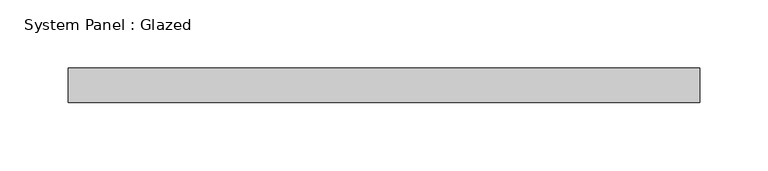
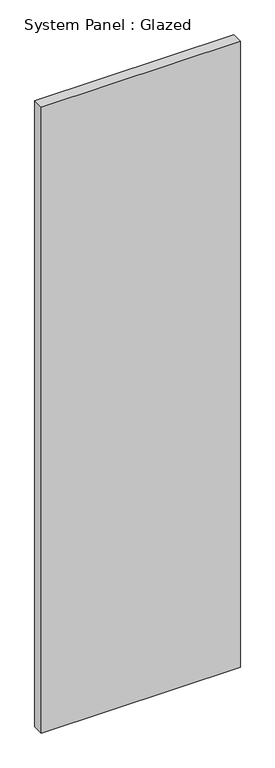
"""IFC4 building model written with IfcOpenShell, lengths in millimetres: plate geometry, System Panel : Glazed."""

from ifc_helpers import new_model, si_unit, origin, origin_with_axes, place, context, project, spatial, polyline, outline, extrude, source, transform, mapped, element, save


def system_panel_glazed_482dc4ba(model_context):
    return source(origin(), model_context, "Body", "SweptSolid", [
        extrude(outline(polyline([(231.775, 19.05), (-231.775, 19.05), (-231.775, 44.45), (231.775, 44.45), (231.775, 19.05)])), origin_with_axes(), (0.0, 0.0, 1.0), 1538.799372),
    ])


if __name__ == "__main__":
    model = new_model("IFC4")
    model_context = context("Model", 3, world=origin())
    ifc_project = project(units=[si_unit("LENGTHUNIT", "METRE", prefix="MILLI")], contexts=[model_context])
    site = spatial("IfcSite", under=ifc_project)
    building = spatial("IfcBuilding", under=site)
    placement = place(None, origin())
    system_panel_glazed_shape = system_panel_glazed_482dc4ba(model_context)
    element("IfcPlate", 1, ObjectType="System Panel : Glazed", at=placement, inside=building, context=model_context, shape_type="MappedRepresentation", body=[
        mapped(system_panel_glazed_shape, transform((0.0, 0.0, 0.0), x_axis=(1.0, 0.0, 0.0), y_axis=(0.0, 1.0, 0.0), z_axis=(0.0, 0.0, 1.0))),
    ])
    save(model, "model.ifc")

# Revit data of these elements
# Type "System Panel : Glazed"
#   Construction Type Id = "GSP4R"
#   Analytic Construction = "1/8 in Pilkington single glazing"
#   Visual Light Transmittance = 0.9
#   Solar Heat Gain Coefficient = 0.86
#   Heat Transfer Coefficient (U) = 1.18115 BTU/(h·ft²·°F)
#   Define Thermal Properties by = 1
# Element 1 (IfcPlate, "System Panel : Glazed")
#   Materials on its faces: "Glass"
# Materials
#   "Glass": class "Glass", colour RGB 0 128 192, transparency 0.75, Description = "Soda Lime Glass", Cost = 0
